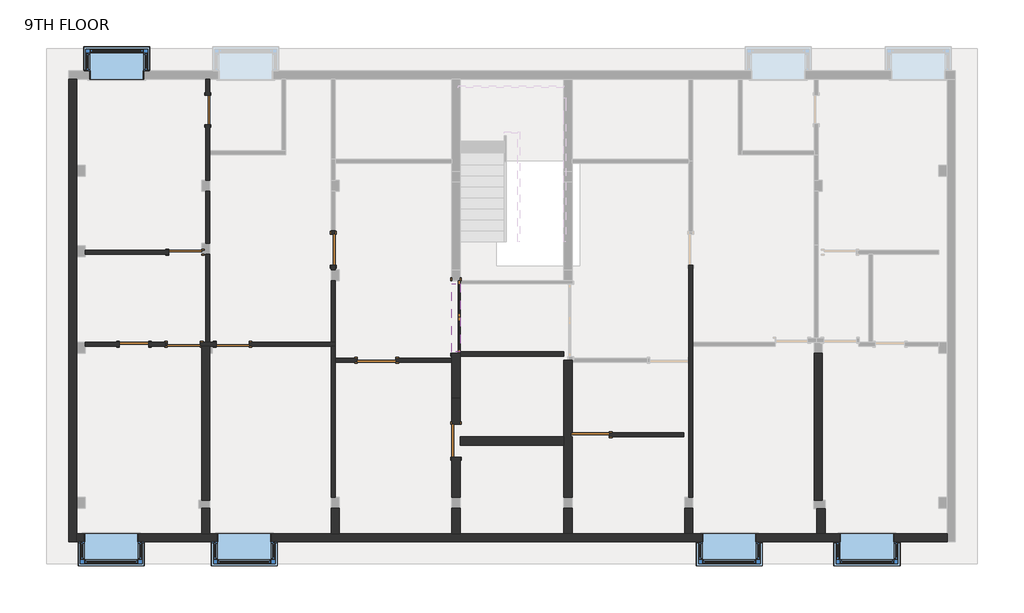
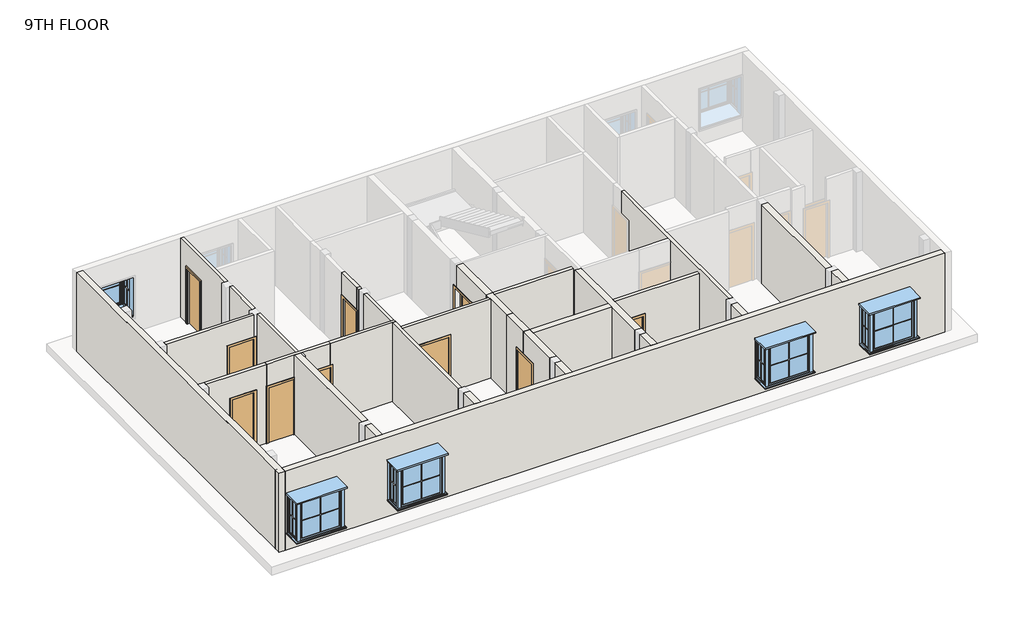
# One storey, part 1 of 3: 32 walls, 10 doors, 5 windows.
"""IFC4 building model written with IfcOpenShell, lengths in millimetres."""

from ifc_helpers import new_model, si_unit, frame, origin, place, context, project, spatial, polyline, outline, extrude, faceted_brep, transform, mapped, element, save
from components import door_77e2dd85, m_door_single_panel_05506f71, m_door_single_panel_3722715f, door_07b5d71c, door_4c0a2014, door_82def9da, m_door_single_panel_3_x7_f8176753, m_door_single_panel_3_x7_ebb67e73, m_door_single_panel_3_x7_ed4aac83, window_19bbd869

model = new_model("IFC4")

# Units and contexts
model_context = context("Model", 3, world=origin())
ifc_project = project(units=[si_unit("LENGTHUNIT", "METRE", prefix="MILLI")], contexts=[model_context])

# Site, building, storey
site = spatial("IfcSite", under=ifc_project)
building = spatial("IfcBuilding", under=site)
storey = spatial("IfcBuildingStorey", under=building, Name="9TH FLOOR", Elevation=32004.0)

# Doors
placement = place(None, origin())
door_shape = door_77e2dd85(model_context)
element("IfcDoor", 1, ObjectType="M_Door-Double-Glass : 6'7\"X7'", at=placement, inside=storey, context=model_context, shape_type="MappedRepresentation", body=[
    mapped(door_shape, transform((-1965.4800498, 1278.6317742, 32004.0), x_axis=(0.0, -1.0, 0.0), y_axis=(1.0, 0.0, 0.0), z_axis=(0.0, 0.0, 1.0))),
])
m_door_single_panel_shape = m_door_single_panel_05506f71(model_context)
element("IfcDoor", 2, ObjectType="M_Door-Single-Panel", at=placement, inside=storey, context=model_context, shape_type="MappedRepresentation", body=[
    mapped(m_door_single_panel_shape, transform((1745.3012085, -1975.7432663, 32004.0), x_axis=(-1.0, 0.0, 0.0), y_axis=(0.0, -1.0, 0.0), z_axis=(0.0, 0.0, 1.0))),
])
m_door_single_panel_2_shape = m_door_single_panel_3722715f(model_context)
element("IfcDoor", 3, ObjectType="M_Door-Single-Panel", at=placement, inside=storey, context=model_context, shape_type="MappedRepresentation", body=[
    mapped(m_door_single_panel_2_shape, transform((-4161.4090098, 90.9578621, 32004.0), x_axis=(-1.0, 0.0, 0.0), y_axis=(0.0, -1.0, 0.0), z_axis=(0.0, 0.0, 1.0))),
])
door_2_shape = door_07b5d71c(model_context)
element("IfcDoor", 4, ObjectType="M_Door-Single-Panel : 2'10\"X7' 2", at=placement, inside=storey, context=model_context, shape_type="MappedRepresentation", body=[
    mapped(door_2_shape, transform((-5360.3487995, 3142.9626891, 32004.0), x_axis=(0.0, -1.0, 0.0), y_axis=(1.0, 0.0, 0.0), z_axis=(0.0, 0.0, 1.0))),
])
door_3_shape = door_4c0a2014(model_context)
element("IfcDoor", 5, ObjectType="M_Door-Single-Panel : 2'8\"X7'", at=placement, inside=storey, context=model_context, shape_type="MappedRepresentation", body=[
    mapped(door_3_shape, transform((-10873.4462614, 526.1567334, 32004.0), x_axis=(1.0, 0.0, 0.0), y_axis=(0.0, 1.0, 0.0), z_axis=(0.0, 0.0, 1.0))),
])
door_4_shape = door_82def9da(model_context)
element("IfcDoor", 6, ObjectType="M_Door-Single-Panel : 2'8\"X7'", at=placement, inside=storey, context=model_context, shape_type="MappedRepresentation", body=[
    mapped(door_4_shape, transform((-8827.4487992, 7008.6751452, 32004.0), x_axis=(0.0, 1.0, 0.0), y_axis=(-1.0, 0.0, 0.0), z_axis=(0.0, 0.0, 1.0))),
])
m_door_single_panel_3_x7_shape = m_door_single_panel_3_x7_f8176753(model_context)
element("IfcDoor", 7, ObjectType="M_Door-Single-Panel : 3'X7'", at=placement, inside=storey, context=model_context, shape_type="MappedRepresentation", body=[
    mapped(m_door_single_panel_3_x7_shape, transform((-9456.0987989, 3078.8567332, 32004.0), x_axis=(1.0, 0.0, 0.0), y_axis=(0.0, 1.0, 0.0), z_axis=(0.0, 0.0, 1.0))),
])
element("IfcDoor", 8, ObjectType="M_Door-Single-Panel : 3'X7'", at=placement, inside=storey, context=model_context, shape_type="MappedRepresentation", body=[
    mapped(m_door_single_panel_3_x7_shape, transform((-8144.8381465, 526.1567334, 32004.0), x_axis=(-1.0, 0.0, 0.0), y_axis=(0.0, -1.0, 0.0), z_axis=(0.0, 0.0, 1.0))),
])
m_door_single_panel_3_x7_2_shape = m_door_single_panel_3_x7_ebb67e73(model_context)
element("IfcDoor", 9, ObjectType="M_Door-Single-Panel : 3'X7'", at=placement, inside=storey, context=model_context, shape_type="MappedRepresentation", body=[
    mapped(m_door_single_panel_3_x7_2_shape, transform((-9494.1987992, 526.1567334, 32004.0), x_axis=(1.0, 0.0, 0.0), y_axis=(0.0, 1.0, 0.0), z_axis=(0.0, 0.0, 1.0))),
])
m_door_single_panel_3_x7_3_shape = m_door_single_panel_3_x7_ed4aac83(model_context)
element("IfcDoor", 10, ObjectType="M_Door-Single-Panel : 3'X7'", at=placement, inside=storey, context=model_context, shape_type="MappedRepresentation", body=[
    mapped(m_door_single_panel_3_x7_3_shape, transform((-1963.0987998, -2146.6357283, 32004.0), x_axis=(0.0, 1.0, 0.0), y_axis=(-1.0, 0.0, 0.0), z_axis=(0.0, 0.0, 1.0))),
])

# Walls
element("IfcWall", 11, ObjectType="4.5\"", at=placement, inside=storey, context=model_context, shape_type="SweptSolid", body=[
    extrude(outline(polyline([(2711.1626891, 35052.0), (3671.8272228, 35052.0), (3671.8272228, 32004.0), (3574.7626891, 32004.0), (3574.7626891, 34137.6), (2711.1626891, 34137.6), (2711.1626891, 35052.0)])), frame((-5417.4987995, 0.0, 0.0), z_axis=(1.0, 0.0, 0.0), x_axis=(0.0, 1.0, 0.0)), (0.0, 0.0, 1.0), 114.3),
])
element("IfcWall", 12, ObjectType="4.5\"", at=placement, inside=storey, context=model_context, shape_type="Brep", body=[
    faceted_brep([(-7690.1644155, 469.0067334, 35052.0), (-8713.148796, 469.0067334, 35052.0), (-8771.750543, 469.0067334, 35052.0), (-9000.350543, 469.0067334, 35052.0), (-10009.8462614, 469.0067334, 35052.0), (-10009.8462614, 469.0067334, 32004.0), (-9951.3987992, 469.0067334, 32004.0), (-9951.3987992, 469.0067334, 34137.6), (-9036.9987992, 469.0067334, 34137.6), (-9036.9987992, 469.0067334, 32004.0), (-9000.350543, 469.0067334, 32004.0), (-8771.750543, 469.0067334, 32004.0), (-8713.148796, 469.0067334, 32004.0), (-8602.0381465, 469.0067334, 32004.0), (-8602.0381465, 469.0067334, 34137.6), (-7690.1644155, 469.0067334, 34137.6), (-10009.8462614, 583.3067334, 35052.0), (-7690.1644155, 583.3067334, 35052.0), (-7690.1644155, 583.3067334, 34137.6), (-8602.0381465, 583.3067334, 34137.6), (-8602.0381465, 583.3067334, 32004.0), (-9036.9987992, 583.3067334, 32004.0), (-9036.9987992, 583.3067334, 34137.6), (-9951.3987992, 583.3067334, 34137.6), (-9951.3987992, 583.3067334, 32004.0), (-10009.8462614, 583.3067334, 32004.0)], [[[0, 1, 2, 3, 4, 5, 6, 7, 8, 9, 10, 11, 12, 13, 14, 15]], [[16, 17, 18, 19, 20, 21, 22, 23, 24, 25]], [[5, 25, 24, 6]], [[9, 21, 20, 13, 12, 11, 10]], [[17, 0, 15, 18]], [[4, 3, 2, 1, 0, 17, 16]], [[5, 4, 16, 25]], [[8, 22, 21, 9]], [[7, 23, 22, 8]], [[23, 7, 6, 24]], [[19, 14, 13, 20]], [[14, 19, 18, 15]]]),
])
element("IfcWall", 13, ObjectType="4.5\"", at=placement, inside=storey, context=model_context, shape_type="SweptSolid", body=[
    extrude(outline(polyline([(32004.0, 4336.1012085), (35052.0, 4336.1012085), (35052.0, 1250.0012085), (34137.6, 1250.0012085), (34137.6, 2278.7012085), (32004.0, 2278.7012085), (32004.0, 4336.1012085)])), frame((0.0, -2032.8932663, 0.0), z_axis=(0.0, 1.0, 0.0), x_axis=(0.0, 0.0, 1.0)), (0.0, 0.0, 1.0), 114.3),
])
element("IfcWall", 14, ObjectType="4.5\"", at=placement, inside=storey, context=model_context, shape_type="Brep", body=[
    faceted_brep([(-1848.7987998, 202.3067742, 32004.0), (1021.4012085, 202.3067742, 32004.0), (1021.4012085, 202.3067742, 35052.0), (-1848.7987998, 202.3067742, 35052.0), (-1848.7987998, 316.6067742, 32004.0), (-1848.7987998, 316.6067742, 34137.6), (-1848.7987998, 316.6067742, 35052.0), (1021.4012085, 316.6067742, 35052.0), (1021.4012085, 316.6067742, 32004.0), (-1848.7987998, 275.3317742, 32004.0)], [[[0, 1, 2, 3]], [[4, 5, 6, 7, 8]], [[1, 0, 9, 4, 8]], [[2, 1, 8, 7]], [[3, 2, 7, 6]], [[0, 3, 6, 5, 4, 9]]]),
])
element("IfcWall", 15, ObjectType="4.5\"", at=placement, inside=storey, context=model_context, shape_type="Brep", body=[
    faceted_brep([(-5417.4987995, 469.0067334, 32004.0), (-5417.4987995, -3709.2932193, 32004.0), (-5417.4987995, -3709.2932193, 35052.0), (-5417.4987995, 469.0067334, 35052.0), (-5303.1987995, 469.0067334, 32004.0), (-5303.1987995, 469.0067334, 35052.0), (-5303.1987995, 148.1078621, 35052.0), (-5303.1987995, 33.8078621, 35052.0), (-5303.1987995, -3709.2932193, 35052.0), (-5303.1987995, -3709.2932193, 32004.0), (-5303.1987995, 33.8078621, 32004.0), (-5303.1987995, 148.1078621, 32004.0)], [[[0, 1, 2, 3]], [[4, 5, 6, 7, 8, 9, 10, 11]], [[1, 0, 4, 11, 10, 9]], [[2, 1, 9, 8]], [[3, 2, 8, 7, 6, 5]], [[0, 3, 5, 4]]]),
])
element("IfcWall", 16, ObjectType="4.5\" 2", at=placement, inside=storey, context=model_context, shape_type="SweptSolid", body=[
    extrude(outline(polyline([(35052.0, -8998.8987989), (35052.0, -12224.6987989), (32004.0, -12224.6987989), (32004.0, -9913.2987989), (34137.6, -9913.2987989), (34137.6, -8998.8987989), (35052.0, -8998.8987989)])), frame((0.0, 3021.7067332, 0.0), z_axis=(0.0, 1.0, 0.0), x_axis=(0.0, 0.0, 1.0)), (0.0, 0.0, 1.0), 114.3),
])
element("IfcWall", 17, ObjectType="4.5\" 2", at=placement, inside=storey, context=model_context, shape_type="SweptSolid", body=[
    extrude(outline(polyline([(-8770.2987992, 4761.606733), (-8770.2987992, 3326.5067332), (-8884.5987992, 3326.5067332), (-8884.5987992, 4761.606733), (-8770.2987992, 4761.606733)])), frame((0.0, 0.0, 32004.0), z_axis=(0.0, 0.0, 1.0), x_axis=(1.0, 0.0, 0.0)), (0.0, 0.0, 1.0), 3048.0),
])
element("IfcWall", 18, ObjectType="4.5\" 2", at=placement, inside=storey, context=model_context, shape_type="Brep", body=[
    faceted_brep([(-8770.2987992, 7415.0751452, 34137.6), (-8770.2987992, 7415.0751452, 32004.0), (-8770.2987992, 7860.4067329, 32004.0), (-8770.2987992, 7860.4067329, 35052.0), (-8770.2987992, 5879.2067329, 35052.0), (-8770.2987992, 5764.9067329, 35052.0), (-8770.2987992, 5066.406733, 35052.0), (-8770.2987992, 5066.406733, 32004.0), (-8770.2987992, 5764.9067329, 32004.0), (-8770.2987992, 5879.2067329, 32004.0), (-8770.2987992, 6602.2751452, 32004.0), (-8770.2987992, 6602.2751452, 34137.6), (-8884.5987992, 7860.4067329, 32004.0), (-8884.5987992, 7415.0751452, 32004.0), (-8884.5987992, 7415.0751452, 34137.6), (-8884.5987992, 6602.2751452, 34137.6), (-8884.5987992, 6602.2751452, 32004.0), (-8884.5987992, 5066.406733, 32004.0), (-8884.5987992, 5066.406733, 35052.0), (-8884.5987992, 7860.4067329, 35052.0)], [[[0, 1, 2, 3, 4, 5, 6, 7, 8, 9, 10, 11]], [[12, 13, 14, 15, 16, 17, 18, 19]], [[2, 1, 13, 12]], [[10, 9, 8, 7, 17, 16]], [[6, 5, 4, 3, 19, 18]], [[7, 6, 18, 17]], [[14, 13, 1, 0]], [[15, 14, 0, 11]], [[16, 15, 11, 10]], [[3, 2, 12, 19]]]),
])
element("IfcWall", 19, ObjectType="4.5\" 2", at=placement, inside=storey, context=model_context, shape_type="SweptSolid", body=[
    extrude(outline(polyline([(34137.6, -10467.0462614), (32004.0, -10467.0462614), (32004.0, -10009.8462614), (35052.0, -10009.8462614), (35052.0, -12224.6987989), (32004.0, -12224.6987989), (32004.0, -11279.8462614), (34137.6, -11279.8462614), (34137.6, -10467.0462614)])), frame((0.0, 469.0067334, 0.0), z_axis=(0.0, 1.0, 0.0), x_axis=(0.0, 0.0, 1.0)), (0.0, 0.0, 1.0), 114.3),
])
element("IfcWall", 20, ObjectType="4.5\" 2", at=placement, inside=storey, context=model_context, shape_type="SweptSolid", body=[
    extrude(outline(polyline([(-8770.298796, 3021.7067332), (-8770.298796, 583.3067804), (-8884.598796, 583.3067804), (-8884.598796, 3021.7067332), (-8770.298796, 3021.7067332)])), frame((0.0, 0.0, 32004.0), z_axis=(0.0, 0.0, 1.0), x_axis=(1.0, 0.0, 0.0)), (0.0, 0.0, 1.0), 3048.0),
])
element("IfcWall", 21, ObjectType="4.5\" 2", at=placement, inside=storey, context=model_context, shape_type="Brep", body=[
    faceted_brep([(-5303.1987995, 469.0067334, 35052.0), (-5417.4987995, 469.0067334, 35052.0), (-7690.1644155, 469.0067334, 35052.0), (-7690.1644155, 469.0067334, 34137.6), (-7687.6381465, 469.0067334, 34137.6), (-7687.6381465, 469.0067334, 32004.0), (-5417.4987995, 469.0067334, 32004.0), (-5303.1987995, 469.0067334, 32004.0), (-7690.1644155, 583.3067334, 35052.0), (-5417.4987995, 583.3067334, 35052.0), (-5303.1987995, 583.3067334, 35052.0), (-5303.1987995, 583.3067334, 32004.0), (-5417.4987995, 583.3067334, 32004.0), (-7687.6381465, 583.3067334, 32004.0), (-7687.6381465, 583.3067334, 34137.6), (-7690.1644155, 583.3067334, 34137.6)], [[[0, 1, 2, 3, 4, 5, 6, 7]], [[8, 9, 10, 11, 12, 13, 14, 15]], [[11, 7, 6, 5, 13, 12]], [[2, 1, 0, 10, 9, 8]], [[2, 8, 15, 3]], [[0, 7, 11, 10]], [[14, 4, 3, 15]], [[4, 14, 13, 5]]]),
])
element("IfcWall", 22, ObjectType="4.5\" 2", at=placement, inside=storey, context=model_context, shape_type="SweptSolid", body=[
    extrude(outline(polyline([(-5303.1987995, 2285.1067802), (-5303.1987995, 583.3067334), (-5417.4987995, 583.3067334), (-5417.4987995, 2285.1067802), (-5303.1987995, 2285.1067802)])), frame((0.0, 0.0, 32004.0), z_axis=(0.0, 0.0, 1.0), x_axis=(1.0, 0.0, 0.0)), (0.0, 0.0, 1.0), 3048.0),
])
element("IfcWall", 23, ObjectType="4.5\" 2", at=placement, inside=storey, context=model_context, shape_type="Brep", body=[
    faceted_brep([(-5303.1987995, 2589.9067802, 32004.0), (-5303.1987995, 2711.1626891, 32004.0), (-5303.1987995, 2711.1626891, 34137.6), (-5303.1987995, 2711.1626891, 35052.0), (-5303.1987995, 2589.9067802, 35052.0), (-5417.4987995, 2589.9067802, 32004.0), (-5417.4987995, 2589.9067802, 35052.0), (-5417.4987995, 2711.1626891, 35052.0), (-5417.4987995, 2711.1626891, 34137.6), (-5417.4987995, 2711.1626891, 32004.0)], [[[0, 1, 2, 3, 4]], [[5, 6, 7, 8, 9]], [[1, 0, 5, 9]], [[3, 2, 1, 9, 8, 7]], [[4, 3, 7, 6]], [[0, 4, 6, 5]]]),
])
element("IfcWall", 24, ObjectType="4.5\" 2", at=placement, inside=storey, context=model_context, shape_type="Brep", body=[
    faceted_brep([(4475.8012082, -3709.2932193, 32004.0), (4475.8012082, -3709.2932193, 35052.0), (4475.8012082, 33.8078621, 35052.0), (4475.8012082, 148.1078621, 35052.0), (4475.8012082, 3132.0737955, 35052.0), (4475.8012082, 3132.0737955, 34137.6), (4475.8012082, 2711.1626891, 34137.6), (4475.8012082, 2711.1626891, 32004.0), (4475.8012082, 148.1078621, 32004.0), (4475.8012082, 33.8078621, 32004.0), (4590.1012082, -3709.2932193, 35052.0), (4590.1012082, -3709.2932193, 32004.0), (4590.1012082, 469.0067334, 32004.0), (4590.1012082, 583.3067334, 32004.0), (4590.1012082, 2711.1626891, 32004.0), (4590.1012082, 2711.1626891, 34137.6), (4590.1012082, 3132.0737955, 34137.6), (4590.1012082, 3132.0737955, 35052.0), (4590.1012082, 583.3067334, 35052.0), (4590.1012082, 469.0067334, 35052.0)], [[[0, 1, 2, 3, 4, 5, 6, 7, 8, 9]], [[10, 11, 12, 13, 14, 15, 16, 17, 18, 19]], [[11, 0, 9, 8, 7, 14, 13, 12]], [[1, 0, 11, 10]], [[4, 3, 2, 1, 10, 19, 18, 17]], [[4, 17, 16, 5]], [[6, 15, 14, 7]], [[15, 6, 5, 16]]]),
])
element("IfcWall", 25, ObjectType="4.5\" 2", at=placement, inside=storey, context=model_context, shape_type="SweptSolid", body=[
    extrude(outline(polyline([(35052.0, -2077.3987998), (35052.0, -5303.1987995), (32004.0, -5303.1987995), (32004.0, -4694.8090098), (34137.6, -4694.8090098), (34137.6, -3628.0090098), (32004.0, -3628.0090098), (32004.0, -2077.3987998), (35052.0, -2077.3987998)])), frame((0.0, 33.8078621, 0.0), z_axis=(0.0, 1.0, 0.0), x_axis=(0.0, 0.0, 1.0)), (0.0, 0.0, 1.0), 114.3),
])
element("IfcWall", 26, ObjectType="9\"", at=placement, inside=storey, context=model_context, shape_type="Brep", body=[
    faceted_brep([(-12453.2987957, -4941.1932661, 32004.0), (-12453.2987957, -4712.5932661, 32004.0), (-12453.2987957, -4014.0932671, 32004.0), (-12453.2987957, -3709.2932671, 32004.0), (-12453.2987957, 278.5067334, 32004.0), (-12453.2987957, 583.3067334, 32004.0), (-12453.2987957, 2951.8567332, 32004.0), (-12453.2987957, 3256.6567332, 32004.0), (-12453.2987957, 5174.3567339, 32004.0), (-12453.2987957, 5479.1567339, 32004.0), (-12453.2987957, 7860.4067329, 32004.0), (-12453.2987957, 7860.4067329, 35052.0), (-12453.2987957, 5479.1567339, 35052.0), (-12453.2987957, 5174.3567339, 35052.0), (-12453.2987957, 3256.6567332, 35052.0), (-12453.2987957, 2951.8567332, 35052.0), (-12453.2987957, 583.3067334, 35052.0), (-12453.2987957, 278.5067334, 35052.0), (-12453.2987957, -3709.2932671, 35052.0), (-12453.2987957, -4014.0932671, 35052.0), (-12453.2987957, -4712.5932661, 35052.0), (-12453.2987957, -4941.1932661, 35052.0), (-12681.8987957, -4941.1932661, 32004.0), (-12681.8987957, -4941.1932661, 35052.0), (-12681.8987957, 7860.4067329, 35052.0), (-12681.8987957, 7860.4067329, 32004.0)], [[[0, 1, 2, 3, 4, 5, 6, 7, 8, 9, 10, 11, 12, 13, 14, 15, 16, 17, 18, 19, 20, 21]], [[22, 23, 24, 25]], [[10, 9, 8, 7, 6, 5, 4, 3, 2, 1, 0, 22, 25]], [[21, 20, 19, 18, 17, 16, 15, 14, 13, 12, 11, 24, 23]], [[11, 10, 25, 24]], [[0, 21, 23, 22]]]),
])
element("IfcWall", 27, ObjectType="9\"", at=placement, inside=storey, context=model_context, shape_type="Brep", body=[
    faceted_brep([(-12453.2987957, -4712.5932661, 32004.0), (-12453.2987957, -4014.0932671, 32004.0), (-12453.2987957, -3709.2932671, 32004.0), (-12453.2987957, 278.5067334, 32004.0), (-12453.2987957, 583.3067334, 32004.0), (-12453.2987957, 2951.8567332, 32004.0), (-12453.2987957, 3256.6567332, 32004.0), (-12453.2987957, 5174.3567339, 32004.0), (-12453.2987957, 5479.1567339, 32004.0), (-12453.2987957, 7860.4067329, 32004.0), (-12453.2987957, 7860.4067329, 35052.0), (-12453.2987957, 5479.1567339, 35052.0), (-12453.2987957, 5174.3567339, 35052.0), (-12453.2987957, 3256.6567332, 35052.0), (-12453.2987957, 2951.8567332, 35052.0), (-12453.2987957, 583.3067334, 35052.0), (-12453.2987957, 278.5067334, 35052.0), (-12453.2987957, -3709.2932671, 35052.0), (-12453.2987957, -4014.0932671, 35052.0), (-12453.2987957, -4712.5932661, 35052.0), (-12681.8987957, -4712.5932661, 32004.0), (-12681.8987957, -4712.5932661, 35052.0), (-12681.8987957, 7860.4067329, 35052.0), (-12681.8987957, 7860.4067329, 32004.0)], [[[0, 1, 2, 3, 4, 5, 6, 7, 8, 9, 10, 11, 12, 13, 14, 15, 16, 17, 18, 19]], [[20, 21, 22, 23]], [[9, 8, 7, 6, 5, 4, 3, 2, 1, 0, 20, 23]], [[19, 18, 17, 16, 15, 14, 13, 12, 11, 10, 22, 21]], [[10, 9, 23, 22]], [[0, 19, 21, 20]]]),
])
element("IfcWall", 28, ObjectType="9\"", at=placement, inside=storey, context=model_context, shape_type="Brep", body=[
    faceted_brep([(-9000.350543, 469.0067334, 32004.0), (-9000.350543, -3785.4932196, 32004.0), (-9000.350543, -3785.4932196, 35052.0), (-9000.350543, 469.0067334, 35052.0), (-8771.750543, 469.0067334, 32004.0), (-8771.750543, 469.0067334, 35052.0), (-8771.750543, 278.5067334, 35052.0), (-8771.750543, -3785.4932196, 35052.0), (-8771.750543, -3785.4932196, 32004.0), (-8771.750543, 278.5067334, 32004.0)], [[[0, 1, 2, 3]], [[4, 5, 6, 7, 8, 9]], [[1, 0, 4, 9, 8]], [[2, 1, 8, 7]], [[3, 2, 7, 6, 5]], [[0, 3, 5, 4]]]),
])
element("IfcWall", 29, ObjectType="9\"", at=placement, inside=storey, context=model_context, shape_type="Brep", body=[
    faceted_brep([(-2077.3987998, -972.2341552, 32004.0), (-2077.3987998, -972.2341552, 35052.0), (-2077.3987998, 33.8078621, 35052.0), (-2077.3987998, 148.1078621, 35052.0), (-2077.3987998, 316.6067742, 35052.0), (-2077.3987998, 316.6067742, 34137.6), (-2077.3987998, 275.3317742, 34137.6), (-2077.3987998, 275.3317742, 32004.0), (-2077.3987998, 148.1078621, 32004.0), (-2077.3987998, 33.8078621, 32004.0), (-1848.7987998, -972.2341552, 35052.0), (-1848.7987998, -972.2341552, 32004.0), (-1848.7987998, 202.3067742, 32004.0), (-1848.7987998, 275.3317742, 32004.0), (-1848.7987998, 275.3317742, 34137.6), (-1848.7987998, 316.6067742, 34137.6), (-1848.7987998, 316.6067742, 35052.0), (-1848.7987998, 202.3067742, 35052.0)], [[[0, 1, 2, 3, 4, 5, 6, 7, 8, 9]], [[10, 11, 12, 13, 14, 15, 16, 17]], [[11, 0, 9, 8, 7, 13, 12]], [[1, 0, 11, 10]], [[4, 3, 2, 1, 10, 17, 16]], [[4, 16, 15, 5]], [[6, 14, 13, 7]], [[14, 6, 5, 15]]]),
])
element("IfcWall", 30, ObjectType="9\"", at=placement, inside=storey, context=model_context, shape_type="Brep", body=[
    faceted_brep([(-2077.3987998, -3709.2932663, 32004.0), (-2077.3987998, -3709.2932663, 35052.0), (-2077.3987998, -2032.3357283, 35052.0), (-2077.3987998, -2032.3357283, 34137.6), (-2077.3987998, -2603.8357283, 34137.6), (-2077.3987998, -2603.8357283, 32004.0), (-1848.7987998, -3709.2932663, 35052.0), (-1848.7987998, -3709.2932663, 32004.0), (-1848.7987998, -2603.8357283, 32004.0), (-1848.7987998, -2603.8357283, 34137.6), (-1848.7987998, -2032.3357283, 34137.6), (-1848.7987998, -2032.3357283, 35052.0), (-1848.7987998, -2260.9357283, 35052.0)], [[[0, 1, 2, 3, 4, 5]], [[6, 7, 8, 9, 10, 11, 12]], [[7, 0, 5, 8]], [[1, 0, 7, 6]], [[2, 1, 6, 12, 11]], [[2, 11, 10, 3]], [[9, 4, 3, 10]], [[4, 9, 8, 5]]]),
])
element("IfcWall", 31, ObjectType="9\"", at=placement, inside=storey, context=model_context, shape_type="Brep", body=[
    faceted_brep([(-1848.7987998, -2260.9357283, 32004.0), (1021.4012085, -2260.9357283, 32004.0), (1021.4012085, -2260.9357283, 35052.0), (-1848.7987998, -2260.9357283, 35052.0), (-1848.7987998, -2032.3357283, 32004.0), (-1848.7987998, -2032.3357283, 34137.6), (-1848.7987998, -2032.3357283, 35052.0), (1021.4012085, -2032.3357283, 35052.0), (1021.4012085, -2032.3357283, 32004.0)], [[[0, 1, 2, 3]], [[4, 5, 6, 7, 8]], [[1, 0, 4, 8]], [[3, 2, 7, 6]], [[2, 1, 8, 7]], [[0, 3, 6, 5, 4]]]),
])
element("IfcWall", 32, ObjectType="9\"", at=placement, inside=storey, context=model_context, shape_type="Brep", body=[
    faceted_brep([(1021.4012085, 90.9578621, 32004.0), (1021.4012085, -2032.3357283, 32004.0), (1021.4012085, -2260.9357283, 32004.0), (1021.4012085, -3709.2932193, 32004.0), (1021.4012085, -3709.2932193, 35052.0), (1021.4012085, -2260.9357283, 35052.0), (1021.4012085, -2032.3357283, 35052.0), (1021.4012085, 90.9578621, 35052.0), (1250.0012085, -3709.2932193, 35052.0), (1250.0012085, -3709.2932193, 32004.0), (1250.0012085, -2032.8932663, 32004.0), (1250.0012085, -2032.8932663, 34137.6), (1250.0012085, -1918.5932663, 34137.6), (1250.0012085, -1918.5932663, 32004.0), (1250.0012085, 33.8078621, 32004.0), (1250.0012085, 90.9578621, 32004.0), (1250.0012085, 90.9578621, 35052.0), (1250.0012085, 33.8078621, 35052.0), (1250.0012085, -1918.5932663, 35052.0), (1250.0012085, -2032.8932663, 35052.0), (1158.0082462, 90.9578621, 32004.0), (1211.9012085, -1918.5932663, 32004.0), (1211.9012085, -2032.8932663, 32004.0), (1158.0082462, 90.9578621, 35052.0), (1211.9012085, -1918.5932663, 34137.6), (1211.9012085, -2032.8932663, 34137.6)], [[[0, 1, 2, 3, 4, 5, 6, 7]], [[8, 9, 10, 11, 12, 13, 14, 15, 16, 17, 18, 19]], [[3, 2, 1, 0, 20, 15, 14, 13, 21, 22, 10, 9]], [[4, 3, 9, 8]], [[7, 6, 5, 4, 8, 19, 18, 17, 16, 23]], [[0, 7, 23, 16, 15, 20]], [[24, 21, 13, 12]], [[22, 25, 11, 10]], [[21, 24, 25, 22]], [[25, 24, 12, 11]]]),
])
element("IfcWall", 33, ObjectType="9\"", at=placement, inside=storey, context=model_context, shape_type="SweptSolid", body=[
    extrude(outline(polyline([(7942.9012047, -3785.4932666), (7942.9012047, 278.5067334), (8171.5012047, 278.5067334), (8171.5012047, -3785.4932666), (7942.9012047, -3785.4932666)])), frame((0.0, 0.0, 32004.0), z_axis=(0.0, 0.0, 1.0), x_axis=(1.0, 0.0, 0.0)), (0.0, 0.0, 1.0), 3048.0),
])
element("IfcWall", 34, ObjectType="9\"", at=placement, inside=storey, context=model_context, shape_type="SweptSolid", body=[
    extrude(outline(polyline([(-1848.7987998, 2196.2067742), (-1848.7987998, 316.6067742), (-2077.3987998, 316.6067742), (-2077.3987998, 2196.2067742), (-1848.7987998, 2196.2067742)])), frame((0.0, 0.0, 34137.6), z_axis=(0.0, 0.0, 1.0), x_axis=(1.0, 0.0, 0.0)), (0.0, 0.0, 1.0), 914.4),
])
element("IfcWall", 35, ObjectType="9\"", at=placement, inside=storey, context=model_context, shape_type="SweptSolid", body=[
    extrude(outline(polyline([(-972.2341552, 35052.0), (-972.2341552, 32004.0), (-1689.4357283, 32004.0), (-1689.4357283, 34137.6), (-2032.3357283, 34137.6), (-2032.3357283, 35052.0), (-972.2341552, 35052.0)])), frame((-2077.3987998, 0.0, 0.0), z_axis=(1.0, 0.0, 0.0), x_axis=(0.0, 1.0, 0.0)), (0.0, 0.0, 1.0), 228.6),
])
element("IfcWall", 36, ObjectType="9\"", at=placement, inside=storey, context=model_context, shape_type="SweptSolid", body=[
    extrude(outline(polyline([(-5417.4987963, -4712.5932661), (-5417.4987963, -4014.0932193), (-5188.8987963, -4014.0932193), (-5188.8987963, -4712.5932661), (-5417.4987963, -4712.5932661)])), frame((0.0, 0.0, 32004.0), z_axis=(0.0, 0.0, 1.0), x_axis=(1.0, 0.0, 0.0)), (0.0, 0.0, 1.0), 3048.0),
])
element("IfcWall", 37, ObjectType="9\"", at=placement, inside=storey, context=model_context, shape_type="SweptSolid", body=[
    extrude(outline(polyline([(4361.5012082, -4712.5932661), (4361.5012082, -4014.0932193), (4590.1012082, -4014.0932193), (4590.1012082, -4712.5932661), (4361.5012082, -4712.5932661)])), frame((0.0, 0.0, 32004.0), z_axis=(0.0, 0.0, 1.0), x_axis=(1.0, 0.0, 0.0)), (0.0, 0.0, 1.0), 3048.0),
])
element("IfcWall", 38, ObjectType="9\"", at=placement, inside=storey, context=model_context, shape_type="SweptSolid", body=[
    extrude(outline(polyline([(-9000.350543, -4712.5932661), (-9000.350543, -4014.0932196), (-8771.750543, -4014.0932196), (-8771.750543, -4712.5932661), (-9000.350543, -4712.5932661)])), frame((0.0, 0.0, 32004.0), z_axis=(0.0, 0.0, 1.0), x_axis=(1.0, 0.0, 0.0)), (0.0, 0.0, 1.0), 3048.0),
])
element("IfcWall", 39, ObjectType="9\"", at=placement, inside=storey, context=model_context, shape_type="SweptSolid", body=[
    extrude(outline(polyline([(-2077.3987998, -4712.5932661), (-2077.3987998, -4014.0932663), (-1848.7987998, -4014.0932663), (-1848.7987998, -4712.5932661), (-2077.3987998, -4712.5932661)])), frame((0.0, 0.0, 32004.0), z_axis=(0.0, 0.0, 1.0), x_axis=(1.0, 0.0, 0.0)), (0.0, 0.0, 1.0), 3048.0),
])
element("IfcWall", 40, ObjectType="9\"", at=placement, inside=storey, context=model_context, shape_type="SweptSolid", body=[
    extrude(outline(polyline([(1021.4012085, -4712.5932661), (1021.4012085, -4014.0932193), (1250.0012085, -4014.0932193), (1250.0012085, -4712.5932661), (1021.4012085, -4712.5932661)])), frame((0.0, 0.0, 32004.0), z_axis=(0.0, 0.0, 1.0), x_axis=(1.0, 0.0, 0.0)), (0.0, 0.0, 1.0), 3048.0),
])
element("IfcWall", 41, ObjectType="9\"", at=placement, inside=storey, context=model_context, shape_type="SweptSolid", body=[
    extrude(outline(polyline([(8017.9646942, -4712.5932661), (8017.9646942, -4015.9914801), (8246.5646942, -4015.9914801), (8246.5646942, -4712.5932661), (8017.9646942, -4712.5932661)])), frame((0.0, 0.0, 32004.0), z_axis=(0.0, 0.0, 1.0), x_axis=(1.0, 0.0, 0.0)), (0.0, 0.0, 1.0), 3048.0),
])
element("IfcWall", 42, ObjectType="9\" 2", at=placement, inside=storey, context=model_context, shape_type="Brep", body=[
    faceted_brep([(-12453.2987957, -4941.1932661, 32004.0), (11625.9012075, -4941.1932662, 32004.0), (11625.9012075, -4941.1932662, 35052.0), (-12453.2987957, -4941.1932661, 35052.0), (8658.6146942, -4941.1932661, 34154.8), (10158.6146942, -4941.1932661, 34154.8), (10158.6146942, -4941.1932661, 32604.0), (8658.6146942, -4941.1932661, 32604.0), (4849.7512082, -4941.1932661, 34154.8), (6349.7512082, -4941.1932661, 34154.8), (6349.7512082, -4941.1932661, 32604.0), (4849.7512082, -4941.1932661, 32604.0), (-8569.250543, -4941.1932661, 34154.8), (-7069.250543, -4941.1932661, 34154.8), (-7069.250543, -4941.1932661, 32604.0), (-8569.250543, -4941.1932661, 32604.0), (-12250.7987957, -4941.1932661, 34154.8), (-10750.7987957, -4941.1932661, 34154.8), (-10750.7987957, -4941.1932661, 32604.0), (-12250.7987957, -4941.1932661, 32604.0), (-12453.2987957, -4712.5932661, 32004.0), (-12453.2987957, -4712.5932661, 35052.0), (-9000.350543, -4712.5932661, 35052.0), (-8771.750543, -4712.5932661, 35052.0), (-5417.4987963, -4712.5932661, 35052.0), (-5188.8987963, -4712.5932661, 35052.0), (-2077.3987998, -4712.5932661, 35052.0), (-1848.7987998, -4712.5932661, 35052.0), (1021.4012085, -4712.5932661, 35052.0), (1250.0012085, -4712.5932661, 35052.0), (4361.5012082, -4712.5932661, 35052.0), (4590.1012082, -4712.5932661, 35052.0), (8017.9646942, -4712.5932661, 35052.0), (8246.5646942, -4712.5932661, 35052.0), (11625.9012075, -4712.5932662, 35052.0), (11625.9012075, -4712.5932662, 32004.0), (8246.5646942, -4712.5932661, 32004.0), (8017.9646942, -4712.5932661, 32004.0), (4590.1012082, -4712.5932661, 32004.0), (4361.5012082, -4712.5932661, 32004.0), (1250.0012085, -4712.5932661, 32004.0), (1021.4012085, -4712.5932661, 32004.0), (-1848.7987998, -4712.5932661, 32004.0), (-2077.3987998, -4712.5932661, 32004.0), (-5188.8987963, -4712.5932661, 32004.0), (-5417.4987963, -4712.5932661, 32004.0), (-8771.750543, -4712.5932661, 32004.0), (-9000.350543, -4712.5932661, 32004.0), (8658.6146942, -4712.5932661, 34154.8), (8658.6146942, -4712.5932661, 32604.0), (10158.6146942, -4712.5932661, 32604.0), (10158.6146942, -4712.5932661, 34154.8), (4849.7512082, -4712.5932661, 34154.8), (4849.7512082, -4712.5932661, 32604.0), (6349.7512082, -4712.5932661, 32604.0), (6349.7512082, -4712.5932661, 34154.8), (-8569.250543, -4712.5932661, 34154.8), (-8569.250543, -4712.5932661, 32604.0), (-7069.250543, -4712.5932661, 32604.0), (-7069.250543, -4712.5932661, 34154.8), (-12250.7987957, -4712.5932661, 34154.8), (-12250.7987957, -4712.5932661, 32604.0), (-10750.7987957, -4712.5932661, 32604.0), (-10750.7987957, -4712.5932661, 34154.8)], [[[0, 1, 2, 3], [4, 5, 6, 7], [8, 9, 10, 11], [12, 13, 14, 15], [16, 17, 18, 19]], [[20, 21, 22, 23, 24, 25, 26, 27, 28, 29, 30, 31, 32, 33, 34, 35, 36, 37, 38, 39, 40, 41, 42, 43, 44, 45, 46, 47], [48, 49, 50, 51], [52, 53, 54, 55], [56, 57, 58, 59], [60, 61, 62, 63]], [[1, 0, 20, 47, 46, 45, 44, 43, 42, 41, 40, 39, 38, 37, 36, 35]], [[3, 2, 34, 33, 32, 31, 30, 29, 28, 27, 26, 25, 24, 23, 22, 21]], [[2, 1, 35, 34]], [[0, 3, 21, 20]], [[49, 48, 4, 7]], [[50, 49, 7, 6]], [[51, 50, 6, 5]], [[48, 51, 5, 4]], [[53, 52, 8, 11]], [[54, 53, 11, 10]], [[55, 54, 10, 9]], [[52, 55, 9, 8]], [[57, 56, 12, 15]], [[58, 57, 15, 14]], [[59, 58, 14, 13]], [[56, 59, 13, 12]], [[61, 60, 16, 19]], [[62, 61, 19, 18]], [[63, 62, 18, 17]], [[60, 63, 17, 16]]]),
])

# Windows
window_shape = window_19bbd869(model_context)
element("IfcWindow", 43, ObjectType="4'.8\"x3'.8\"", at=placement, inside=storey, context=model_context, shape_type="MappedRepresentation", body=[
    mapped(window_shape, transform((-11500.7987957, -4826.8932661, 32004.0), x_axis=(-1.0, 0.0, 0.0), y_axis=(0.0, -1.0, 0.0), z_axis=(0.0, 0.0, 1.0))),
])
element("IfcWindow", 44, ObjectType="4'.8\"x3'.8\"", at=placement, inside=storey, context=model_context, shape_type="MappedRepresentation", body=[
    mapped(window_shape, transform((-7819.250543, -4826.8932661, 32004.0), x_axis=(-1.0, 0.0, 0.0), y_axis=(0.0, -1.0, 0.0), z_axis=(0.0, 0.0, 1.0))),
])
element("IfcWindow", 45, ObjectType="4'.8\"x3'.8\"", at=placement, inside=storey, context=model_context, shape_type="MappedRepresentation", body=[
    mapped(window_shape, transform((5599.7512082, -4826.8932661, 32004.0), x_axis=(-1.0, 0.0, 0.0), y_axis=(0.0, -1.0, 0.0), z_axis=(0.0, 0.0, 1.0))),
])
element("IfcWindow", 46, ObjectType="4'.8\"x3'.8\"", at=placement, inside=storey, context=model_context, shape_type="MappedRepresentation", body=[
    mapped(window_shape, transform((9408.6146942, -4826.8932661, 32004.0), x_axis=(-1.0, 0.0, 0.0), y_axis=(0.0, -1.0, 0.0), z_axis=(0.0, 0.0, 1.0))),
])
element("IfcWindow", 47, ObjectType="4'.8\"x3'.8\"", at=placement, inside=storey, context=model_context, shape_type="MappedRepresentation", body=[
    mapped(window_shape, transform((-11348.3987957, 7974.7067329, 32004.0), x_axis=(1.0, 0.0, 0.0), y_axis=(0.0, 1.0, 0.0), z_axis=(0.0, 0.0, 1.0))),
])

save(model, "model.ifc")

# Revit data of these elements
# Type "M_Door-Double-Glass : 6'7\"X7'"
#   Type Mark = "16"
#   Construction Type Id = "opn-d45"
#   Assembly Code = "C1020"
#   Analytic Construction = "Wood frame, double glass door "
#   W = 3' - 3 1/2"
#   Thickness = 0' - 1.9685"
#   Thermal Resistance (R) = 1.8150 (h·ft²·°F)/BTU
#   Swing Angle [instance default] = 90.00°
#   Heat Transfer Coefficient (U) = 0.5510 BTU/(h·ft²·°F)
#   Height = 7' - 0"
#   Bottom Rail = 0' - 3.93701"
#   Top Rail = 0' - 3.93701"
#   Stiles = 0' - 3.93701"
#   Trim Projection = 0' - 0.98425"
#   Trim Width = 0' - 3.14961"
#   Width = 6' - 7"
#   Define Thermal Properties by = 1
#   Glazing = Glass
#   Panel Material = Wood - Birch - Solid Stained Light Low Gloss
#   Trim Material = Paint - Sienna
#   Visual Light Transmittance = 0
#   Solar Heat Gain Coefficient = 0
#   Function = (empty or 0)
#   Wall Closure = (empty or 0)
# Type "M_Door-Single-Panel"
#   Type Mark = "14"
#   Construction Type Id = "DOOR"
#   Assembly Code = "C1020300"
#   Analytic Construction = "Wooden"
#   Thickness = 0' - 1.9685"
#   Thermal Resistance (R) = 2.5876 (h·ft²·°F)/BTU
#   Swing Angle [instance default] = 90.00°
#   Heat Transfer Coefficient (U) = 0.3865 BTU/(h·ft²·°F)
#   Height = 7' - 0"
#   Trim Projection Ext = 0' - 0.98425"
#   Trim Projection Int = 0' - 0.98425"
#   Trim Width = 0' - 3.14961"
#   Width = 3' - 6"
#   Define Thermal Properties by = 1
#   Panel Material = Wood - Birch - Solid Stained Light Low Gloss
#   Trim Material = Paint - Sienna
#   Visual Light Transmittance = 0
#   Solar Heat Gain Coefficient = 0
#   Function = (empty or 0)
#   Wall Closure = (empty or 0)
# Type "M_Door-Single-Panel : 2'10\"X7' 2"
#   Type Mark = "10"
#   Construction Type Id = "DOOR"
#   Assembly Code = "C1020300"
#   Analytic Construction = "Wooden"
#   Thickness = 0' - 1.9685"
#   Thermal Resistance (R) = 2.5876 (h·ft²·°F)/BTU
#   Swing Angle [instance default] = 90.00°
#   Heat Transfer Coefficient (U) = 0.3865 BTU/(h·ft²·°F)
#   Height = 7' - 0"
#   Trim Projection Ext = 0' - 0.98425"
#   Trim Projection Int = 0' - 0.98425"
#   Trim Width = 0' - 3.14961"
#   Width = 2' - 10"
#   Define Thermal Properties by = 1
#   Panel Material = Wood - Birch - Solid Stained Light Low Gloss
#   Trim Material = Paint - Sienna
#   Visual Light Transmittance = 0
#   Solar Heat Gain Coefficient = 0
#   Function = (empty or 0)
#   Wall Closure = (empty or 0)
# Type "M_Door-Single-Panel : 2'8\"X7'"
#   Type Mark = "9"
#   Construction Type Id = "DOOR"
#   Assembly Code = "C1020300"
#   Analytic Construction = "Wooden"
#   Thickness = 0' - 1.9685"
#   Thermal Resistance (R) = 2.5876 (h·ft²·°F)/BTU
#   Swing Angle [instance default] = 90.00°
#   Heat Transfer Coefficient (U) = 0.3865 BTU/(h·ft²·°F)
#   Height = 7' - 0"
#   Trim Projection Ext = 0' - 0.98425"
#   Trim Projection Int = 0' - 0.98425"
#   Trim Width = 0' - 3.14961"
#   Width = 2' - 8"
#   Define Thermal Properties by = 1
#   Panel Material = Wood - Birch - Solid Stained Light Low Gloss
#   Trim Material = Paint - Sienna
#   Visual Light Transmittance = 0
#   Solar Heat Gain Coefficient = 0
#   Function = (empty or 0)
#   Wall Closure = (empty or 0)
# Type "M_Door-Single-Panel : 3'X7'"
#   Type Mark = "11"
#   Construction Type Id = "DOOR"
#   Assembly Code = "C1020300"
#   Analytic Construction = "Wooden"
#   Thickness = 0' - 1.9685"
#   Thermal Resistance (R) = 2.5876 (h·ft²·°F)/BTU
#   Swing Angle [instance default] = 90.00°
#   Heat Transfer Coefficient (U) = 0.3865 BTU/(h·ft²·°F)
#   Height = 7' - 0"
#   Trim Projection Ext = 0' - 0.98425"
#   Trim Projection Int = 0' - 0.98425"
#   Trim Width = 0' - 3.14961"
#   Width = 3' - 0"
#   Define Thermal Properties by = 1
#   Panel Material = Wood - Birch - Solid Stained Light Low Gloss
#   Trim Material = Paint - Sienna
#   Visual Light Transmittance = 0
#   Solar Heat Gain Coefficient = 0
#   Function = (empty or 0)
#   Wall Closure = (empty or 0)
# Type "4.5\""
#   Assembly Code = "B2010"
#   Layers, outside or top first: 0' - 4 1/2" no material (function 1)
# Type "4.5\" 2"
#   Assembly Code = "B2010"
#   Layers, outside or top first: 0' - 4 1/2" no material (function 1)
# Type "9\""
#   Assembly Code = "B2010"
#   Layers, outside or top first: 0' - 9" no material (function 1)
# Type "9\" 2"
#   Assembly Code = "B2010"
#   Layers, outside or top first: 0' - 9" no material (function 1)
# Type "4'.8\"x3'.8\""
#   Type Mark = "20"
#   Fire Rating = "0.5h"
#   Assembly Code = "B2020100"
#   Analytic Construction = "1/8 in Pilkington single glazing"
#   Width = 4' - 11.05512"
#   Wall Thickness [instance default] = 0' - 5.90551"
#   Visual Light Transmittance = 0.9
#   Trim Width = 5' - 7.05512"
#   Trim Height = 4' - 11.05512"
#   Thermal Resistance (R) = 1.5394 (h·ft²·°F)/BTU
#   Solar Heat Gain Coefficient = 0.86
#   Rough Width = 4' - 11.64567"
#   Rough Height = 4' - 11.64567"
#   Height 1 = 5' - 1.05512"
#   Height = 4' - 11.05512"
#   Heat Transfer Coefficient (U) = 0.6496 BTU/(h·ft²·°F)
#   Depth = 1' - 11.62205"
#   Default Sill Height = 1' - 11.62205"
#   Side Muntin Visibility = yes
#   Center Muntin Visibility = yes
#   Interior Trim Visibility [instance default] = yes
#   Exterior Trim Visibility [instance default] = yes
#   Side Muntin Pattern = M_Muntin Pattern_2x2 : M_Muntin Pattern_2x2
#   Center Muntin Pattern = M_Muntin Pattern_2x2 : M_Muntin Pattern_2x2
#   Interior Trim Material = Wood - Stained
#   Exterior Trim Material = Clad - White
#   Exterior Trim = element 422966
#   Interior Trim = M_Trim-Window-Interior-Flat : Picture Frame
#   Interior Frame Material = Wood - Stained
#   Glass Panel Material = Glass
#   Exterior Frame Material = Clad - White
#   Wall Closure = (empty or 0)
# Element 1 (IfcDoor, "M_Door-Double-Glass : 6'7\"X7'")
#   Swing Angle = 90.00°
#   Phase Created = New Construction
#   Materials on its faces: "Wood - Birch - Solid Stained Light Low Gloss", "Paint - Sienna", "Glass"
# Elements 2, 3 (IfcDoor, "M_Door-Single-Panel")
#   Swing Angle = 90.00°
#   Phase Created = New Construction
#   Materials on its faces: "Paint - Sienna", "Wood - Birch - Solid Stained Light Low Gloss"
# Element 4 (IfcDoor, "M_Door-Single-Panel : 2'10\"X7' 2")
#   Swing Angle = 90.00°
#   Phase Created = New Construction
#   Materials on its faces: "Paint - Sienna", "Wood - Birch - Solid Stained Light Low Gloss"
# Elements 5, 6 (IfcDoor, "M_Door-Single-Panel : 2'8\"X7'")
#   Swing Angle = 90.00°
#   Phase Created = New Construction
#   Materials on its faces: "Paint - Sienna", "Wood - Birch - Solid Stained Light Low Gloss"
# Elements 7, 8, 9, 10 (IfcDoor, "M_Door-Single-Panel : 3'X7'")
#   Swing Angle = 90.00°
#   Phase Created = New Construction
#   Materials on its faces: "Paint - Sienna", "Wood - Birch - Solid Stained Light Low Gloss"
# Elements 11, 12, 13, 14, 15 (IfcWall, "4.5\"")
#   Top Offset = -0' - 6"
#   Base Offset = 0' - 0"
#   wall height = 10' - 0"
#   Phase Created = New Construction
#   Base Constraint = 9TH FLOOR
#   Top Constraint = 10 TH FLOOR
#   Materials on its faces: "Default Wall"
# Elements 16, 17, 18, 19, 20, 21, 22, 23, 24, 25 (IfcWall, "4.5\" 2")
#   Top Offset = -0' - 6"
#   Base Offset = 0' - 0"
#   wall height = 10' - 0"
#   Phase Created = New Construction
#   Base Constraint = 9TH FLOOR
#   Top Constraint = 10 TH FLOOR
#   Materials on its faces: "Default Wall"
# Elements 26, 27, 28, 29, 30, 31, 32, 33, 34, 35, 36, 37, 38, 39, 40, 41 (IfcWall, "9\"")
#   Top Offset = -0' - 6"
#   Base Offset = 0' - 0"
#   wall height = 10' - 0"
#   Phase Created = New Construction
#   Base Constraint = 9TH FLOOR
#   Top Constraint = 10 TH FLOOR
#   Materials on its faces: "Default Wall"
# Element 42 (IfcWall, "9\" 2")
#   Top Offset = -0' - 6"
#   Base Offset = 0' - 0"
#   wall height = 10' - 0"
#   Phase Created = New Construction
#   Base Constraint = 9TH FLOOR
#   Top Constraint = 10 TH FLOOR
#   Materials on its faces: "Default Wall"
# Element 43 (IfcWindow, "4'.8\"x3'.8\"")
#   Mark = "247"
#   Interior Trim Visibility = yes
#   Exterior Trim Visibility = yes
#   Phase Created = New Construction
#   Materials on its faces: "Clad - White", "Wood - Stained", "Glass"
# Element 44 (IfcWindow, "4'.8\"x3'.8\"")
#   Mark = "248"
#   Interior Trim Visibility = yes
#   Exterior Trim Visibility = yes
#   Phase Created = New Construction
#   Materials on its faces: "Clad - White", "Wood - Stained", "Glass"
# Element 45 (IfcWindow, "4'.8\"x3'.8\"")
#   Mark = "249"
#   Interior Trim Visibility = yes
#   Exterior Trim Visibility = yes
#   Phase Created = New Construction
#   Materials on its faces: "Clad - White", "Wood - Stained", "Glass"
# Element 46 (IfcWindow, "4'.8\"x3'.8\"")
#   Mark = "250"
#   Interior Trim Visibility = yes
#   Exterior Trim Visibility = yes
#   Phase Created = New Construction
#   Materials on its faces: "Clad - White", "Wood - Stained", "Glass"
# Element 47 (IfcWindow, "4'.8\"x3'.8\"")
#   Mark = "291"
#   Interior Trim Visibility = yes
#   Exterior Trim Visibility = yes
#   Phase Created = New Construction
#   Materials on its faces: "Clad - White", "Wood - Stained", "Glass"
# Materials
#   "Glass": class "Glass", colour RGB 0 128 192, transparency 0.75, Description = "Soda Lime Glass", Cost = 0
#   "Wood - Birch - Solid Stained Light Low Gloss": class "Wood", colour RGB 210 159 95, transparency 0, Cost = 0
#   "Paint - Sienna": colour RGB 118 70 51, transparency 0, Cost = 0
#   "Wood - Stained": class "Wood", colour RGB 224 178 126, transparency 0, Cost = 0
#   "Clad - White": class "Wood", colour RGB 242 242 238, transparency 0, Cost = 0
#   "Default Wall": colour RGB 128 128 128, transparency 0, Cost = 0
